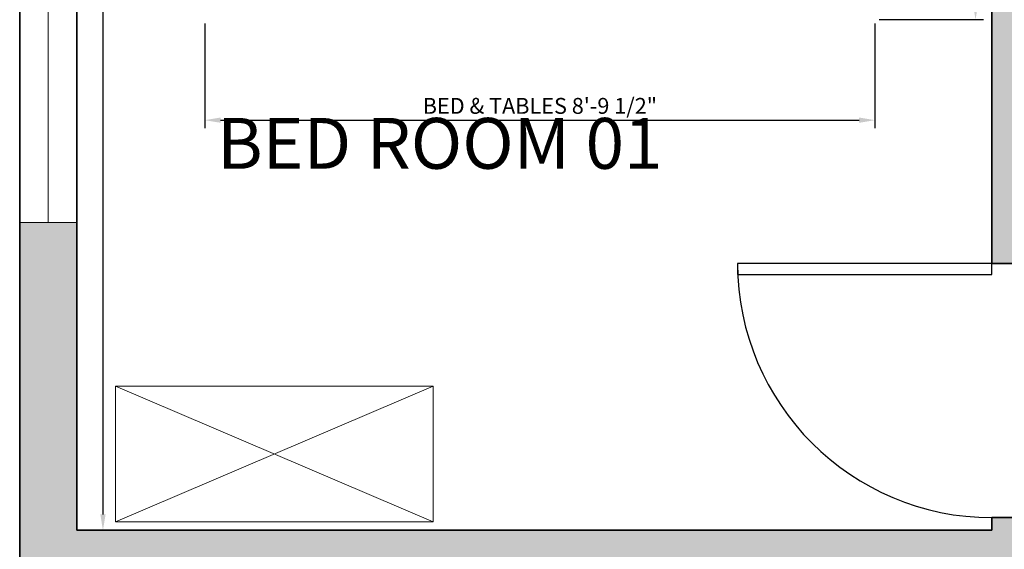
# Model space of a CAD drawing. Units: inches. Extents: x 2901 to 5923, y 918 to 2827.
# Tile 4 of 16: x 4430 to 4585, y 1450 to 1534. Entities that reach past the tile are written whole.
import ezdxf

# ---------------------------------------------------------------- set-up
doc = ezdxf.new("R2010")
doc.units = ezdxf.units.IN
for name, color, linetype, lineweight in [('A-ANNO-DIMS', 2, 'Continuous', 18), ('A-AREA-IDEN', 7, 'Continuous', 25), ('A-GLAZ', 4, 'Continuous', 18), ('A-WALL-PATT', 7, 'Continuous', 13), ('doors', 240, 'Continuous', 25), ('furniture', 160, 'Continuous', 18), ('walls', 7, 'Continuous', 35)]:
    doc.layers.add(name, color=color, linetype=linetype, lineweight=lineweight)
doc.styles.get("Standard").update_dxf_attribs({"font": 'arial.ttf'})
doc.dimstyles.new('Copy of ISO-25', dxfattribs={"dimtxt": 2.5, "dimasz": 2.5, "dimexe": 1.25, "dimexo": 0.625, "dimtad": 1, "dimdec": 1, "dimlunit": 4, "dimtxsty": 'Standard', "dimcen": 2.5, "dimadec": 0, "dimazin": 0, "dimtfac": 1, "dimtdec": 1, "dimtmove": 0, "dimatfit": 3, "dimfxl": 1, "dimarcsym": 0})

# ---------------------------------------------------------------- blocks, each defined once
blk = doc.blocks.new('*U5')
for p, q in [((0, 0), (0, -6)), ((-40, 0), (-40, -6))]:
    blk.add_line(p, q)
blk.add_lwpolyline([(0, 0), (0, 40), (-1.75, 40), (-1.75, 0)], close=True)
blk.add_arc((0, 0), 40, 90, 180)
blk = doc.blocks.new('*U19')
for p, q in [((0, 0), (38, 89)), ((38, 0), (0, 89))]:
    blk.add_line(p, q)
blk.add_lwpolyline([(0, 0), (38, 0), (38, 89), (0, 89)], close=True)
blk = doc.blocks.new('*D27')
at = {"layer": 'A-ANNO-DIMS', "color": 0, "lineweight": -2, "transparency": 16777216}
for p, q in [((4429.44, 1621.4), (4424.64, 1621.4)), ((4425.89, 1618.9), (4425.89, 1248.9)), ((4429.44, 1246.4), (4424.64, 1246.4))]:
    blk.add_line(p, q, dxfattribs=at)
at = {"layer": 'A-ANNO-DIMS', "color": 0, "transparency": 16777216}
for points in [[(4425.47, 1618.9), (4426.31, 1618.9), (4425.89, 1621.4)], [(4425.47, 1248.9), (4426.31, 1248.9), (4425.89, 1246.4)]]:
    blk.add_solid(points, dxfattribs=at)
at = {"layer": 'Defpoints', "color": 0, "transparency": 16777216}
for p in [(4430.07, 1621.4), (4425.89, 1246.4), (4430.07, 1246.4)]:
    blk.add_point(p, dxfattribs=at)
at = {"layer": 'A-ANNO-DIMS', "color": 0, "transparency": 16777216, "insert": (4423.99, 1433.9), "char_height": 2.5, "attachment_point": 5, "rotation": 90}
blk.add_mtext('31\'-3"', dxfattribs=at)
blk = doc.blocks.new('*D40')
at = {"layer": 'A-ANNO-DIMS', "color": 0, "lineweight": -2, "transparency": 16777216}
for p, q in [((4439.69, 1621.4), (4444.42, 1621.4)), ((4443.17, 1618.9), (4443.17, 1455.9)), ((4439.69, 1453.4), (4444.42, 1453.4))]:
    blk.add_line(p, q, dxfattribs=at)
at = {"layer": 'A-ANNO-DIMS', "color": 0, "transparency": 16777216}
for points in [[(4442.76, 1618.9), (4443.59, 1618.9), (4443.17, 1621.4)], [(4442.76, 1455.9), (4443.59, 1455.9), (4443.17, 1453.4)]]:
    blk.add_solid(points, dxfattribs=at)
at = {"layer": 'Defpoints', "color": 0, "transparency": 16777216}
for p in [(4439.07, 1621.4), (4439.07, 1453.4), (4443.17, 1453.4)]:
    blk.add_point(p, dxfattribs=at)
at = {"layer": 'A-ANNO-DIMS', "color": 0, "transparency": 16777216, "insert": (4441.29, 1537.4), "char_height": 2.5, "attachment_point": 5, "rotation": 90}
blk.add_mtext("14'", dxfattribs=at)
blk = doc.blocks.new('*D81')
at = {"layer": 'A-ANNO-DIMS', "color": 0, "lineweight": -2, "transparency": 16777216}
for p, q in [((4459.19, 1533.17), (4459.19, 1516.72)), ((4564.68, 1533.17), (4564.68, 1516.72)), ((4461.69, 1517.97), (4562.18, 1517.97))]:
    blk.add_line(p, q, dxfattribs=at)
at = {"layer": 'A-ANNO-DIMS', "color": 0, "transparency": 16777216}
for points in [[(4461.69, 1518.39), (4461.69, 1517.56), (4459.19, 1517.97)], [(4562.18, 1518.39), (4562.18, 1517.56), (4564.68, 1517.97)]]:
    blk.add_solid(points, dxfattribs=at)
at = {"layer": 'Defpoints', "color": 0, "transparency": 16777216}
for p in [(4459.19, 1533.8), (4564.68, 1533.8), (4564.68, 1517.97)]:
    blk.add_point(p, dxfattribs=at)
at = {"layer": 'A-ANNO-DIMS', "color": 0, "transparency": 16777216, "insert": (4511.94, 1519.9), "char_height": 2.5, "attachment_point": 5}
blk.add_mtext('BED & TABLES 8\'-9 1/2"', dxfattribs=at)
blk = doc.blocks.new('*D82')
at = {"layer": 'A-ANNO-DIMS', "color": 0, "lineweight": -2, "transparency": 16777216}
for p, q in [((4565.31, 1616.24), (4581.76, 1616.24)), ((4580.51, 1536.3), (4580.51, 1613.74)), ((4565.31, 1533.8), (4581.76, 1533.8))]:
    blk.add_line(p, q, dxfattribs=at)
at = {"layer": 'A-ANNO-DIMS', "color": 0, "transparency": 16777216}
for points in [[(4580.09, 1613.74), (4580.92, 1613.74), (4580.51, 1616.24)], [(4580.09, 1536.3), (4580.92, 1536.3), (4580.51, 1533.8)]]:
    blk.add_solid(points, dxfattribs=at)
at = {"layer": 'Defpoints', "color": 0, "transparency": 16777216}
for p in [(4564.68, 1616.24), (4580.51, 1616.24), (4564.68, 1533.8)]:
    blk.add_point(p, dxfattribs=at)
at = {"layer": 'A-ANNO-DIMS', "color": 0, "transparency": 16777216, "insert": (4578.59, 1575.02), "char_height": 2.5, "attachment_point": 5, "rotation": 90}
blk.add_mtext('6\'-10 1/2"', dxfattribs=at)

msp = doc.modelspace()

# ---------------------------------------------------------------- hatches: boundary and pattern name
at = {"layer": 'A-WALL-PATT'}
h = msp.add_hatch(color=256, dxfattribs=at)
h.dxf.hatch_style = 1
h.paths.add_polyline_path([(4439.07, 1447.4), (4583.07, 1447.4), (4583.07, 1340.4), (4589.07, 1340.4), (4589.07, 1453.4), (4589.07, 1455.39), (4583.07, 1455.39), (4583.07, 1453.4), (4439.07, 1453.4), (4439.07, 1501.84), (4430.07, 1501.84), (4430.07, 1399.4), (4439.07, 1399.4)])
h.paths.add_polyline_path([(4439.07, 1621.4), (4487.07, 1621.4), (4487.07, 1630.4), (4430.07, 1630.4), (4430.07, 1561.84), (4439.07, 1561.84)])
h.paths.add_polyline_path([(4630.61, 1630.4), (4535.07, 1630.4), (4535.07, 1621.4), (4583.07, 1621.4), (4583.07, 1495.4), (4589.07, 1495.4), (4637.07, 1495.4), (4637.07, 1501.4), (4589.07, 1501.4), (4589.07, 1621.4), (4630.61, 1621.4)])
h.paths.add_polyline_path([(4892.07, 1630.4), (4690.61, 1630.4), (4690.61, 1621.4), (4733.07, 1621.4), (4733.07, 1564.4), (4739.07, 1564.4), (4739.07, 1621.4), (4883.07, 1621.4), (4883.07, 1528.4), (4739.07, 1528.4), (4733.07, 1528.4), (4733.07, 1501.4), (4685.07, 1501.4), (4685.07, 1495.4), (4739.07, 1495.4), (4739.07, 1519.4), (4787.07, 1519.4), (4787.07, 1423.4), (4739.07, 1423.4), (4739.07, 1456.67), (4733.07, 1456.67), (4733.07, 1340.4), (4739.07, 1340.4), (4739.07, 1417.4), (4787.07, 1417.4), (4793.07, 1417.4), (4793.07, 1423.4), (4793.07, 1519.4), (4883.07, 1519.4), (4883.07, 1482.87), (4892.07, 1482.87)])
h.paths.add_polyline_path([(4892.07, 1458.87), (4883.07, 1458.87), (4883.07, 1423.4), (4823.07, 1423.4), (4823.07, 1417.4), (4883.07, 1417.4), (4883.07, 1363.31), (4892.07, 1363.31)], flags=17)
h.paths.add_polyline_path([(4892.07, 1303.31), (4883.07, 1303.31), (4883.07, 1255.4), (4739.07, 1255.4), (4739.07, 1304.4), (4733.07, 1304.4), (4733.07, 1303.4), (4733.07, 1297.4), (4733.07, 1255.4), (4733.07, 1248.4), (4811.07, 1248.4), (4811.07, 1212.16), (4820.07, 1212.16), (4820.07, 1248.4), (4892.07, 1248.4)])
h.paths.add_polyline_path([(4820.07, 1182.16), (4811.07, 1182.16), (4811.07, 1152.4), (4685.07, 1152.4), (4685.07, 1147.03), (4685.07, 1143.4), (4733.07, 1143.4), (4811.07, 1143.4), (4814.07, 1143.4), (4820.07, 1143.4)])
h.paths.add_polyline_path([(4637.07, 1152.4), (4589.07, 1152.4), (4589.07, 1153.4), (4583.86, 1153.4), (4583.07, 1153.4), (4583.07, 1152.4), (4511.07, 1152.4), (4511.07, 1182.16), (4502.07, 1182.16), (4502.07, 1143.4), (4568.07, 1143.4), (4583.07, 1143.4), (4583.07, 1023.4), (4739.07, 1023.4), (4739.07, 1143.4), (4733.07, 1143.4), (4733.07, 1029.4), (4589.07, 1029.4), (4589.07, 1143.4), (4637.07, 1143.4), (4637.07, 1146.97)])
h.paths.add_polyline_path([(4511.07, 1246.4), (4583.07, 1246.4), (4583.07, 1188.4), (4589.07, 1188.4), (4589.07, 1246.4), (4589.07, 1248.4), (4589.07, 1255.4), (4589.07, 1297.4), (4697.07, 1297.4), (4697.07, 1303.4), (4589.07, 1303.4), (4589.07, 1304.4), (4583.07, 1304.4), (4583.07, 1255.4), (4439.07, 1255.4), (4439.07, 1261.4), (4439.07, 1351.4), (4430.07, 1351.4), (4430.07, 1252.4), (4430.07, 1246.4), (4439.07, 1246.4), (4487.07, 1246.4), (4502.07, 1246.4), (4502.07, 1212.16), (4511.07, 1212.16)])

# ---------------------------------------------------------------- linework, layer by layer
at = {"layer": 'A-GLAZ'}
for p, q in [((4430.07, 1561.84), (4430.07, 1501.84)), ((4434.57, 1561.84), (4434.57, 1501.84)), ((4430.07, 1501.84), (4439.07, 1501.84))]:
    msp.add_line(p, q, dxfattribs=at)
at = {"layer": 'walls'}
for p, q in [((4583.07, 1621.4), (4583.07, 1495.4)), ((4589.07, 1495.4), (4583.07, 1495.4)), ((4589.07, 1455.4), (4583.07, 1455.4)), ((4583.07, 1455.4), (4583.07, 1453.4)), ((4583.07, 1453.4), (4439.07, 1453.4))]:
    msp.add_line(p, q, dxfattribs=at)
for points in [[(4892.07, 1630.4), (4430.07, 1630.4), (4430.07, 1252.4)], [(4583.07, 1621.4), (4439.07, 1621.4), (4439.07, 1453.4)]]:
    msp.add_lwpolyline(points, dxfattribs=at)

# ---------------------------------------------------------------- block references
at = {"layer": 'doors', "xscale": 1.000274864133266, "yscale": 1.000274864133266, "zscale": 1.000274864133266, "rotation": 90}
msp.add_blockref('*U5', (4583.07, 1495.4), dxfattribs=at)
at = {"layer": 'furniture', "xscale": 0.5619183198370973, "yscale": 0.5619183198370973, "zscale": 0.5619183198370973, "rotation": 89.99999999999999}
msp.add_blockref('*U19', (4495.14, 1454.75), dxfattribs=at)

# ---------------------------------------------------------------- texts
at = {"layer": 'A-AREA-IDEN'}
msp.add_text('BED ROOM 01', height=8, dxfattribs=at).set_placement((4461.14, 1510.32))

# ---------------------------------------------------------------- dimensions: what is measured, and where the dimension line sits
at = {"layer": 'A-ANNO-DIMS'}
for base, p1, p2, override, picture, middle in [((4425.89, 1246.4), (4430.07, 1621.4), (4430.07, 1246.4), {"dimclrd": 0, "dimclre": 0, "dimclrt": 0}, '*D27', (4423.99, 1433.9)), ((4443.17, 1453.4), (4439.07, 1621.4), (4439.07, 1453.4), {"dimclrd": 0, "dimclre": 0, "dimclrt": 0}, '*D40', (4441.29, 1537.4)), ((4580.51, 1616.24), (4564.68, 1533.8), (4564.68, 1616.24), {"dimdec": 1, "dimlfac": 1, "dimrnd": 0, "dimzin": 1, "dimdsep": 46, "dimlunit": 4, "dimfrac": 2}, '*D82', (4578.59, 1575.02))]:
    dim = msp.add_linear_dim(base=base, p1=p1, p2=p2, angle=90, dimstyle='Copy of ISO-25', override=override, dxfattribs=at)
    dim.commit()
    dim.dimension.update_dxf_attribs({"geometry": picture, "text_midpoint": middle})
dim = msp.add_linear_dim(base=(4564.68, 1517.97), p1=(4459.19, 1533.8), p2=(4564.68, 1533.8), text='BED & TABLES <>', dimstyle='Copy of ISO-25', override={"dimdec": 1, "dimlfac": 1, "dimrnd": 0, "dimzin": 1, "dimdsep": 46, "dimlunit": 4, "dimfrac": 2}, dxfattribs=at)
dim.commit()
dim.dimension.update_dxf_attribs({"geometry": '*D81', "text_midpoint": (4511.94, 1519.9)})

doc.saveas('drawing.dxf')
